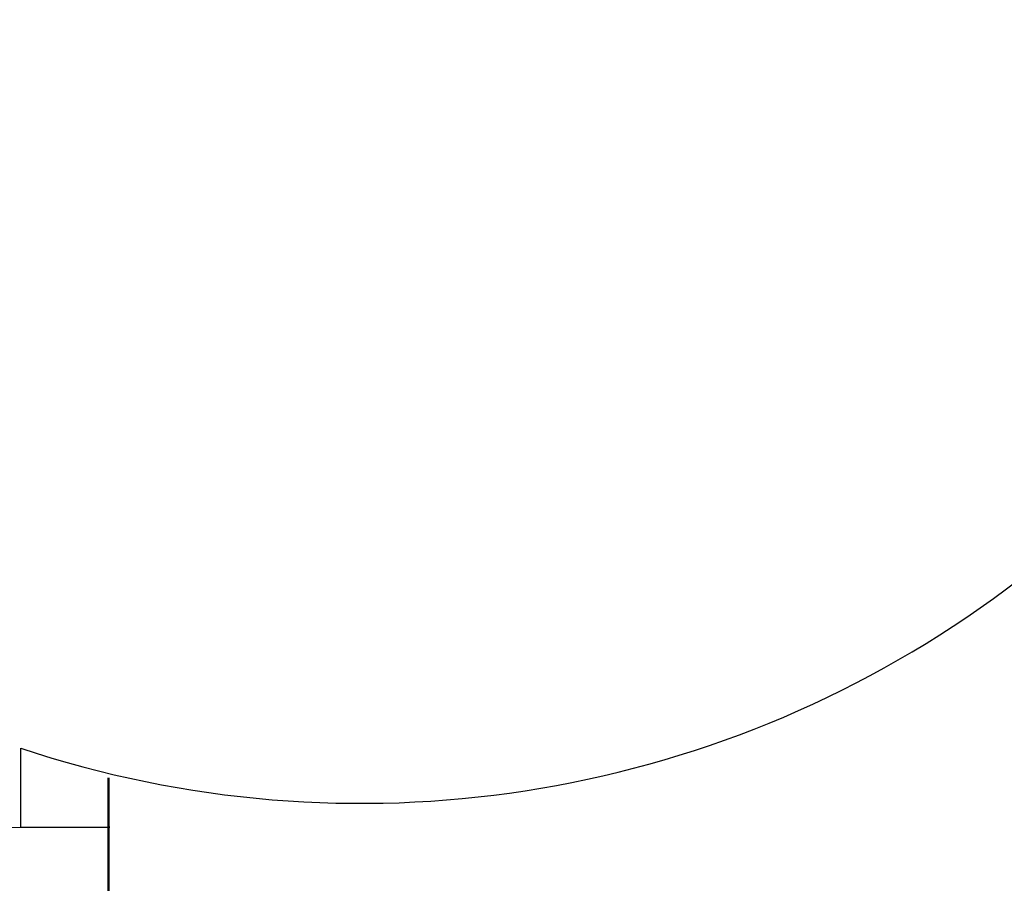
# Model space of a CAD drawing. Units: inches. Extents: x 963 to 2075, y 289 to 2657.
# Tile 8 of 98: x 1374 to 1399, y 1675 to 1696. Entities that reach past the tile are written whole.
import ezdxf

# ---------------------------------------------------------------- set-up
doc = ezdxf.new("R2010")
doc.units = ezdxf.units.IN
for name, color, linetype, lineweight in [('A-DOOR', 4, 'Continuous', 25), ('A-WALL', 7, 'Continuous', 50), ('A-WALL-PATT', 8, 'Continuous', 13)]:
    doc.layers.add(name, color=color, linetype=linetype, lineweight=lineweight)

# ---------------------------------------------------------------- blocks, each defined once
blk = doc.blocks.new('DOOR-5')
for p, q in [((0, 38.25), (0, 33.75)), ((0, 33.75), (0, 36)), ((0, 36), (2, 36))]:
    blk.add_line(p, q)
blk.add_arc((27.907, 27.321), 27.321, 161.4794, 270)

msp = doc.modelspace()

# ---------------------------------------------------------------- hatches: boundary and pattern name
at = {"layer": 'A-WALL-PATT'}
h = msp.add_hatch(dxfattribs=at)
h.set_pattern_fill('ANSI32', color=256)
h.paths.add_polyline_path([(1910.422, 1929.422), (1910.422, 1963.511), (1905.922, 1963.511), (1905.922, 1929.422), (1845.922, 1929.422), (1845.922, 1993.365), (1843.672, 1993.365), (1841.422, 1993.365), (1841.422, 1951.163), (1841.422, 1924.922), (1853.422, 1924.922), (1853.422, 1913.074), (1857.922, 1913.074), (1857.922, 1924.922), (1910.422, 1924.922)])
h.paths.add_polyline_path([(1857.922, 1853.074), (1853.422, 1853.074), (1853.422, 1826.318), (1841.422, 1826.318), (1674.482, 1826.318), (1674.482, 1821.818), (1853.422, 1821.818), (1857.922, 1821.818)])
h.paths.add_polyline_path([(1857.922, 1821.818), (1853.422, 1821.818), (1853.422, 1807.793), (1857.922, 1807.793)])
h.paths.add_polyline_path([(1857.922, 1747.793), (1853.422, 1747.793), (1853.422, 1713.818), (1809.343, 1713.818), (1809.343, 1709.318), (1905.922, 1709.318), (1905.922, 1688.318), (1910.422, 1688.318), (1910.422, 1713.818), (1857.922, 1713.818)])
h.paths.add_polyline_path([(1830.922, 1542.818), (1837.429, 1542.818), (1837.429, 1545.068), (1837.429, 1547.318), (1823.419, 1547.318), (1823.419, 1545.068), (1823.419, 1542.818), (1826.422, 1542.818), (1826.422, 1482.818), (1742.422, 1482.818), (1742.422, 1505.389), (1737.922, 1505.389), (1737.922, 1478.318), (1830.922, 1478.318)])
h.paths.add_polyline_path([(1938.922, 1619.318), (1934.422, 1619.318), (1910.422, 1619.318), (1910.422, 1628.318), (1908.172, 1628.318), (1905.922, 1628.318), (1905.922, 1614.818), (1934.422, 1614.818), (1934.422, 1547.318), (1905.922, 1547.318), (1899.589, 1547.318), (1899.589, 1542.818), (1910.422, 1542.818), (1938.922, 1542.818)])
h.paths.add_polyline_path([(1803.676, 1547.318), (1773.922, 1547.318), (1773.922, 1709.318), (1777.757, 1709.318), (1777.757, 1713.818), (1701.922, 1713.818), (1701.922, 1697.802), (1706.422, 1697.802), (1706.422, 1709.318), (1769.422, 1709.318), (1769.422, 1662.818), (1706.422, 1662.818), (1706.422, 1674.385), (1701.922, 1674.385), (1701.922, 1662.818), (1675.672, 1662.818), (1675.672, 1658.318), (1769.422, 1658.318), (1769.422, 1547.318), (1729.17, 1547.318), (1729.17, 1542.818), (1737.922, 1542.818), (1737.922, 1529.389), (1742.422, 1529.389), (1742.422, 1542.818), (1803.676, 1542.818)])
h.paths.add_polyline_path([(1595.422, 1542.818), (1599.245, 1542.818), (1599.245, 1547.318), (1584.36, 1547.318), (1584.36, 1542.818), (1590.922, 1542.818), (1590.922, 1436.318), (1595.422, 1436.318), (1595.422, 1440.818)])
h.paths.add_polyline_path([(1693.17, 1547.318), (1649.422, 1547.318), (1649.422, 1658.318), (1652.098, 1658.318), (1652.098, 1660.568), (1652.098, 1662.818), (1649.422, 1662.818), (1649.422, 1680.937), (1647.172, 1680.937), (1644.922, 1680.937), (1644.922, 1547.318), (1622.422, 1547.318), (1622.422, 1545.068), (1622.422, 1542.818), (1649.422, 1542.818), (1679.422, 1542.818), (1679.422, 1529.845), (1681.672, 1529.845), (1683.922, 1529.845), (1683.922, 1542.818), (1693.17, 1542.818), (1693.17, 1545.068)])
h.paths.add_polyline_path([(1683.922, 1505.845), (1679.422, 1505.845), (1679.422, 1483.805), (1595.422, 1483.805), (1595.422, 1479.305), (1683.922, 1479.305)])
h.paths.add_polyline_path([(1402.993, 1547.318), (1376.422, 1547.318), (1376.422, 1675.888), (1374.172, 1675.888), (1371.922, 1675.888), (1371.922, 1662.818), (1368.876, 1662.818), (1368.876, 1658.318), (1371.922, 1658.318), (1371.922, 1547.318), (1335.464, 1547.318), (1335.464, 1542.818), (1337.422, 1542.818), (1337.422, 1526.732), (1341.922, 1526.732), (1341.922, 1542.818), (1371.922, 1542.818), (1402.993, 1542.818)])

# ---------------------------------------------------------------- linework, layer by layer
at = {"layer": 'A-WALL'}
msp.add_line((1376.422, 1677.258), (1376.422, 1547.318), dxfattribs=at)

# ---------------------------------------------------------------- block references
at = {"layer": 'A-DOOR', "rotation": 90.14142652708767}
msp.add_blockref('DOOR-5', (1410.204, 1676.091), dxfattribs=at)

doc.saveas('drawing.dxf')
